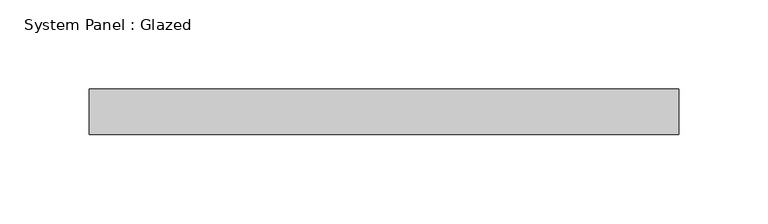
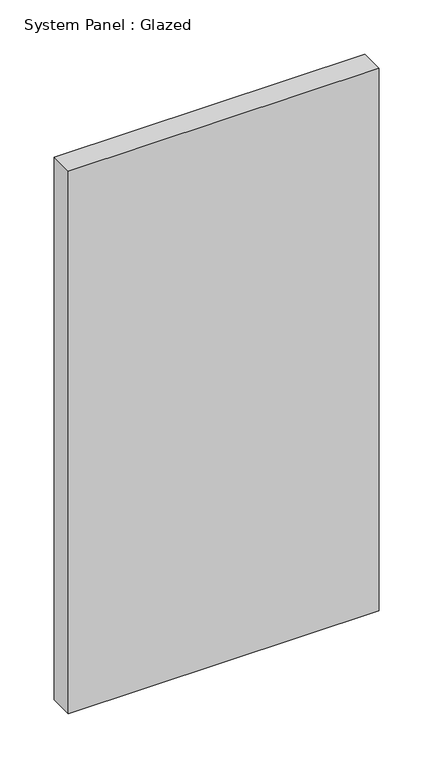
"""IFC4 building model written with IfcOpenShell, lengths in millimetres: plate geometry, System Panel : Glazed."""

from ifc_helpers import new_model, si_unit, origin, origin_with_axes, place, context, project, spatial, polyline, outline, extrude, source, transform, mapped, element, save


def system_panel_glazed_e5302343(model_context):
    return source(origin(), model_context, "Body", "SweptSolid", [
        extrude(outline(polyline([(165.1, 19.05), (-165.1, 19.05), (-165.1, 44.45), (165.1, 44.45), (165.1, 19.05)])), origin_with_axes(), (0.0, 0.0, 1.0), 609.2285299),
    ])


if __name__ == "__main__":
    model = new_model("IFC4")
    model_context = context("Model", 3, world=origin())
    ifc_project = project(units=[si_unit("LENGTHUNIT", "METRE", prefix="MILLI")], contexts=[model_context])
    site = spatial("IfcSite", under=ifc_project)
    building = spatial("IfcBuilding", under=site)
    placement = place(None, origin())
    system_panel_glazed_shape = system_panel_glazed_e5302343(model_context)
    element("IfcPlate", 1, ObjectType="System Panel : Glazed", at=placement, inside=building, context=model_context, shape_type="MappedRepresentation", body=[
        mapped(system_panel_glazed_shape, transform((0.0, 0.0, 0.0), x_axis=(1.0, 0.0, 0.0), y_axis=(0.0, 1.0, 0.0), z_axis=(0.0, 0.0, 1.0))),
    ])
    save(model, "model.ifc")

# Revit data of these elements
# Type "System Panel : Glazed"
#   Construction Type Id = "GSP4R"
#   Analytic Construction = "1/8 in Pilkington single glazing"
#   Visual Light Transmittance = 0.9
#   Solar Heat Gain Coefficient = 0.86
#   Heat Transfer Coefficient (U) = 1.18115 BTU/(h·ft²·°F)
#   Define Thermal Properties by = 1
# Element 1 (IfcPlate, "System Panel : Glazed")
#   Materials on its faces: "Glass"
# Materials
#   "Glass": class "Glass", colour RGB 0 128 192, transparency 0.75, Description = "Soda Lime Glass", Cost = 0
